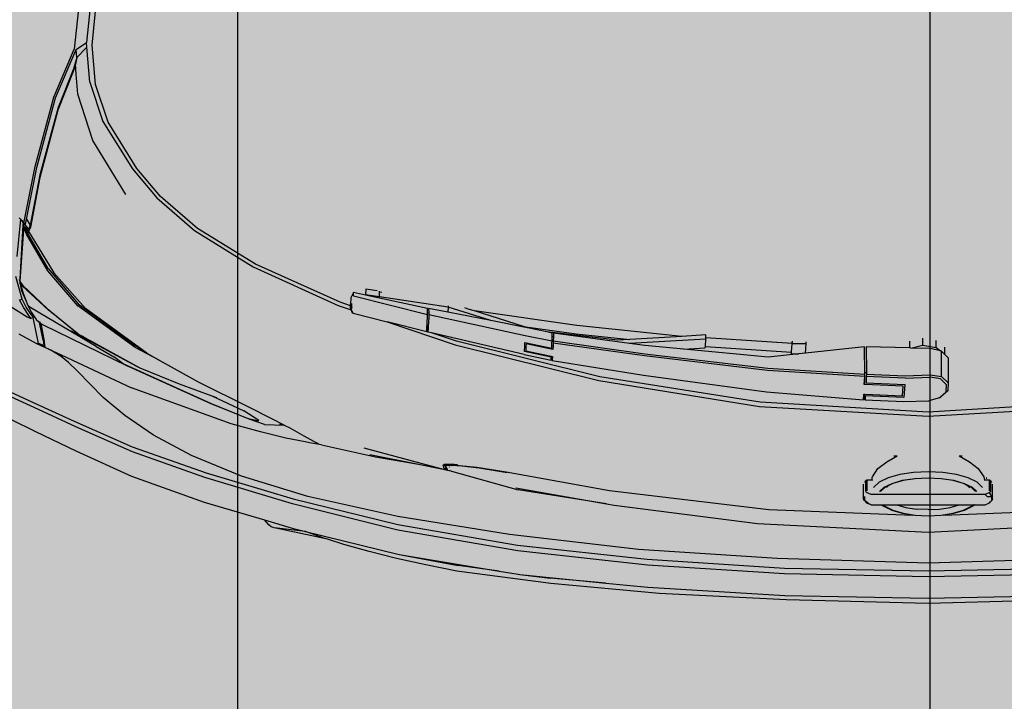
# Model space of a CAD drawing. Units: inches. Extents: x 1884 to 2398, y 474 to 1488.
# Tile 5 of 39: x 2203 to 2232, y 577 to 597. Entities that reach past the tile are written whole.
import ezdxf

# ---------------------------------------------------------------- set-up
doc = ezdxf.new("R2010")
doc.units = ezdxf.units.IN
doc.header["$MEASUREMENT"] = 0
doc.layers.get('0').update_dxf_attribs({"color": 250})
doc.layers.add('A-ANNO-DIMS', color=2, linetype='Continuous', lineweight=18)
doc.layers.add('C-VEHI', color=8, linetype='Continuous', lineweight=18)
doc.layers.add('Edges', color=250, linetype='Continuous')
doc.layers.add('L-PVMT-PATT', color=9, linetype='Continuous', lineweight=13, true_color=0xc7c8ca)
doc.styles.get("Standard").update_dxf_attribs({"font": 'arial.ttf'})
doc.dimstyles.get("Standard").update_dxf_attribs({"dimtxt": 7, "dimasz": 0.18, "dimexe": 0.18, "dimexo": 0.0625, "dimgap": 0.09, "dimtad": 0, "dimtih": 1, "dimtoh": 1, "dimzin": 0, "dimdsep": 46, "dimlunit": 3, "dimtxsty": 'Standard', "dimcen": 0.09, "dimadec": 0, "dimazin": 0, "dimtfac": 1, "dimtofl": 0, "dimtmove": 0, "dimatfit": 3, "dimfxl": 1, "dimtolj": 1, "dimtzin": 0, "dimarcsym": 0})

# ---------------------------------------------------------------- blocks, each defined once
blk = doc.blocks.new('Nissan Qashqai pl')
at = {"layer": 'Edges'}
for p, q in [((11.5166, 12.04708), (11.52386, 11.92208)), ((11.52698, 11.92208), (11.51964, 12.0475)), ((11.61327, 11.92208), (11.60675, 12.04892)), ((11.60051, 11.93346), (11.59629, 12.04057)), ((11.63292, 12.0344), (11.63628, 11.92208)), ((11.64211, 11.92208), (11.63993, 12.02899)), ((11.64437, 12.02886), (11.64655, 11.92208)), ((11.66226, 11.92208), (11.66041, 12.02874)), ((11.66349, 12.02738), (11.66628, 11.92208)), ((11.57479, 11.96843), (11.57457, 11.96768)), ((11.58239, 11.96768), (11.57457, 11.96768)), ((11.57457, 11.96768), (11.57457, 11.96395)), ((11.57617, 11.96938), (11.57479, 11.96843)), ((11.57479, 11.96843), (11.58262, 11.96843)), ((11.58846, 11.97008), (11.57758, 11.97008)), ((11.58262, 11.96843), (11.58377, 11.96782)), ((11.58668, 11.96947), (11.58377, 11.96782)), ((11.58377, 11.96782), (11.58513, 11.96453)), ((11.58679, 11.96604), (11.58668, 11.96947)), ((11.58961, 11.96947), (11.58668, 11.96947)), ((11.58846, 11.97008), (11.58961, 11.96947)), ((11.5915, 11.96782), (11.58961, 11.96947)), ((11.5915, 11.96782), (11.59043, 11.96839)), ((11.59285, 11.96453), (11.5915, 11.96782)), ((11.56082, 11.95281), (11.56588, 11.95938)), ((11.56588, 11.95938), (11.57195, 11.96347)), ((11.57195, 11.96347), (11.57457, 11.96395)), ((11.57261, 11.96533), (11.57261, 11.96561)), ((11.57306, 11.96528), (11.57306, 11.96569)), ((11.57457, 11.96395), (11.57457, 11.96378)), ((11.57994, 11.96265), (11.57613, 11.95845)), ((11.58679, 11.96604), (11.58513, 11.96453)), ((11.58513, 11.96453), (11.58513, 11.87963)), ((11.59285, 11.95694), (11.59285, 11.96453)), ((11.55816, 11.94815), (11.56082, 11.95281)), ((11.57286, 11.95178), (11.57035, 11.94308)), ((11.57613, 11.95845), (11.57286, 11.95178)), ((11.57692, 11.94885), (11.57987, 11.95487)), ((11.57876, 11.95169), (11.57712, 11.94834)), ((11.58001, 11.95424), (11.57876, 11.95169)), ((11.57876, 11.95169), (11.57995, 11.953)), ((11.57987, 11.95487), (11.58291, 11.95821)), ((11.58291, 11.95743), (11.58001, 11.95424)), ((11.59285, 11.95694), (11.59412, 11.95487)), ((11.59285, 11.95657), (11.59285, 11.95694)), ((11.59319, 11.9559), (11.59285, 11.95657)), ((11.59285, 11.95626), (11.59285, 11.95657)), ((11.59285, 11.95626), (11.59319, 11.9559)), ((11.59285, 11.95549), (11.59285, 11.95626)), ((11.59398, 11.95424), (11.59285, 11.95549)), ((11.59285, 11.94526), (11.59285, 11.95549)), ((11.59319, 11.9559), (11.59412, 11.95487)), ((11.59688, 11.94834), (11.59398, 11.95424)), ((11.59412, 11.95487), (11.59707, 11.94885)), ((11.55654, 11.94509), (11.55639, 11.94749)), ((11.55654, 11.94509), (11.55816, 11.94815)), ((11.57466, 11.94101), (11.57692, 11.94885)), ((11.57712, 11.94834), (11.5749, 11.94065)), ((11.59285, 11.8989), (11.59285, 11.94526)), ((11.59478, 11.93858), (11.59285, 11.94526)), ((11.5991, 11.94065), (11.59688, 11.94834)), ((11.59707, 11.94885), (11.59933, 11.94101)), ((11.48349, 11.93703), (11.48106, 11.93457)), ((11.48349, 11.93703), (11.50222, 11.93704)), ((11.49744, 11.93207), (11.50222, 11.93704)), ((11.50222, 11.93704), (11.50812, 11.93671)), ((11.57035, 11.94308), (11.56877, 11.93295)), ((11.57324, 11.93188), (11.57466, 11.94101)), ((11.5749, 11.94065), (11.5735, 11.93169)), ((11.59602, 11.93062), (11.59478, 11.93858)), ((11.60049, 11.93169), (11.5991, 11.94065)), ((11.59933, 11.94101), (11.60051, 11.93346)), ((11.48106, 11.93457), (11.47554, 11.93456)), ((11.47578, 11.92803), (11.4784, 11.93124)), ((11.4784, 11.93124), (11.47657, 11.92368)), ((11.4786, 11.93206), (11.4784, 11.93124)), ((11.48106, 11.93457), (11.4786, 11.93206)), ((11.49744, 11.93207), (11.4786, 11.93206)), ((11.49621, 11.92369), (11.49744, 11.93207)), ((11.49907, 11.93132), (11.49795, 11.92364)), ((11.50349, 11.93588), (11.49907, 11.93132)), ((11.50889, 11.93558), (11.50349, 11.93588)), ((11.50812, 11.93671), (11.51287, 11.9312)), ((11.50889, 11.93558), (11.51321, 11.93053)), ((11.51321, 11.93053), (11.51287, 11.9312)), ((11.51321, 11.93053), (11.51543, 11.92267)), ((11.56877, 11.93295), (11.56823, 11.92208)), ((11.57275, 11.92208), (11.57324, 11.93188)), ((11.5735, 11.93169), (11.57302, 11.92208)), ((11.59645, 11.92208), (11.59602, 11.93062)), ((11.60097, 11.92208), (11.60049, 11.93169)), ((11.60051, 11.93346), (11.60076, 11.93188)), ((11.60076, 11.93188), (11.60124, 11.92208)), ((11.47578, 11.92803), (11.47062, 11.92803)), ((11.47398, 11.91798), (11.47578, 11.92803)), ((11.47657, 11.92368), (11.47622, 11.90912)), ((11.49689, 11.90495), (11.49621, 11.92369)), ((11.49859, 11.9049), (11.49795, 11.92364)), ((11.51606, 11.90392), (11.51543, 11.92267)), ((11.46896, 11.91798), (11.47398, 11.91798)), ((11.47622, 11.90912), (11.47398, 11.91798)), ((11.52386, 11.92208), (11.5166, 11.79708)), ((11.51964, 11.79666), (11.52698, 11.92208)), ((11.56823, 11.92208), (11.56877, 11.91121)), ((11.57324, 11.91228), (11.57275, 11.92208)), ((11.57302, 11.92208), (11.5735, 11.91247)), ((11.59645, 11.92208), (11.59602, 11.91354)), ((11.60049, 11.91247), (11.60097, 11.92208)), ((11.60124, 11.92208), (11.60076, 11.91228)), ((11.60675, 11.79524), (11.61327, 11.92208)), ((11.63628, 11.92208), (11.63292, 11.80976)), ((11.63993, 11.81518), (11.64211, 11.92208)), ((11.64655, 11.92208), (11.64437, 11.8153)), ((11.66041, 11.81542), (11.66226, 11.92208)), ((11.66628, 11.92208), (11.66349, 11.81678)), ((11.47102, 11.90825), (11.4762, 11.90826)), ((11.4762, 11.90826), (11.47542, 11.87608)), ((11.47622, 11.90912), (11.4762, 11.90826)), ((11.56877, 11.91121), (11.57035, 11.90108)), ((11.57466, 11.90315), (11.57324, 11.91228)), ((11.5735, 11.91247), (11.5749, 11.90351)), ((11.59478, 11.90558), (11.59602, 11.91354)), ((11.59629, 11.80359), (11.60051, 11.91071)), ((11.5991, 11.90351), (11.60049, 11.91247)), ((11.60051, 11.91071), (11.59933, 11.90315)), ((11.60076, 11.91228), (11.60051, 11.91071)), ((11.49565, 11.87616), (11.49689, 11.90495)), ((11.49859, 11.9049), (11.49735, 11.87612)), ((11.50223, 11.8759), (11.50346, 11.90468)), ((11.50462, 11.90341), (11.50341, 11.87505)), ((11.50346, 11.90468), (11.51299, 11.90415)), ((11.51177, 11.90301), (11.50462, 11.90341)), ((11.51058, 11.87508), (11.51177, 11.90301)), ((11.51299, 11.90415), (11.51176, 11.87537)), ((11.51483, 11.87514), (11.51606, 11.90392)), ((11.57035, 11.90108), (11.57286, 11.89238)), ((11.57692, 11.89531), (11.57466, 11.90315)), ((11.5749, 11.90351), (11.57712, 11.89582)), ((11.59285, 11.8989), (11.59478, 11.90558)), ((11.59688, 11.89582), (11.5991, 11.90351)), ((11.59933, 11.90315), (11.59707, 11.89531)), ((11.55639, 11.89667), (11.55654, 11.89907)), ((11.55816, 11.89601), (11.55654, 11.89907)), ((11.56082, 11.89135), (11.55816, 11.89601)), ((11.57987, 11.88929), (11.57692, 11.89531)), ((11.57712, 11.89582), (11.57876, 11.89248)), ((11.59285, 11.88868), (11.59285, 11.8989)), ((11.59398, 11.88992), (11.59688, 11.89582)), ((11.59707, 11.89531), (11.59412, 11.88929)), ((11.56588, 11.88478), (11.56082, 11.89135)), ((11.57286, 11.89238), (11.57613, 11.88571)), ((11.57995, 11.89116), (11.57876, 11.89248)), ((11.57876, 11.89248), (11.58001, 11.88992)), ((11.58291, 11.88595), (11.57987, 11.88929)), ((11.58001, 11.88992), (11.58291, 11.88673)), ((11.59285, 11.88868), (11.59398, 11.88992)), ((11.59285, 11.88722), (11.59412, 11.88929)), ((11.59285, 11.8879), (11.59285, 11.88868)), ((11.59285, 11.88759), (11.59319, 11.88827)), ((11.59319, 11.88827), (11.59285, 11.8879)), ((11.59285, 11.88759), (11.59285, 11.8879)), ((11.59285, 11.88722), (11.59285, 11.88759)), ((11.59285, 11.87963), (11.59285, 11.88722)), ((11.59412, 11.88929), (11.59319, 11.88827)), ((11.57195, 11.88069), (11.56588, 11.88478)), ((11.57261, 11.88057), (11.57195, 11.88069)), ((11.57261, 11.88057), (11.57261, 11.88076)), ((11.57306, 11.88049), (11.57261, 11.88057)), ((11.57306, 11.88049), (11.57306, 11.88081)), ((11.57457, 11.88021), (11.57306, 11.88049)), ((11.57457, 11.88096), (11.57457, 11.88021)), ((11.57457, 11.88021), (11.57457, 11.87648)), ((11.57613, 11.88571), (11.57994, 11.88151)), ((11.58513, 11.87963), (11.58377, 11.87635)), ((11.59285, 11.87963), (11.59221, 11.87812)), ((11.49563, 11.87496), (11.47539, 11.87488)), ((11.47539, 11.87488), (11.4801, 11.83099)), ((11.47542, 11.87608), (11.49451, 11.87616)), ((11.49133, 11.80278), (11.49563, 11.87496)), ((11.49732, 11.87492), (11.49295, 11.80271)), ((11.49449, 11.87502), (11.49451, 11.87616)), ((11.50341, 11.87505), (11.49449, 11.87502)), ((11.49451, 11.87616), (11.49565, 11.87616)), ((11.49732, 11.87492), (11.49563, 11.87496)), ((11.49565, 11.87616), (11.49735, 11.87612)), ((11.50339, 11.87463), (11.49732, 11.87492)), ((11.49735, 11.87612), (11.50223, 11.8759)), ((11.50341, 11.87505), (11.50339, 11.87463)), ((11.50884, 11.80182), (11.5148, 11.87394)), ((11.51054, 11.87423), (11.51058, 11.87508)), ((11.5148, 11.87394), (11.51054, 11.87423)), ((11.51472, 11.8751), (11.51058, 11.87508)), ((11.51176, 11.87537), (11.51472, 11.87515)), ((11.51472, 11.87515), (11.51472, 11.8751)), ((11.51472, 11.87515), (11.51483, 11.87514)), ((11.51483, 11.87514), (11.51472, 11.8751)), ((11.57457, 11.87648), (11.58239, 11.87648)), ((11.57457, 11.87648), (11.57479, 11.87573)), ((11.58262, 11.87573), (11.57479, 11.87573)), ((11.57479, 11.87573), (11.57617, 11.87478)), ((11.58846, 11.87408), (11.57758, 11.87408)), ((11.58377, 11.87635), (11.58262, 11.87573)), ((11.58668, 11.87469), (11.58961, 11.87469)), ((11.58961, 11.87469), (11.58846, 11.87408)), ((11.58961, 11.87469), (11.5915, 11.87635)), ((11.59043, 11.87577), (11.58961, 11.87469)), ((11.59221, 11.87812), (11.59043, 11.87577)), ((11.59043, 11.87577), (11.5915, 11.87635)), ((11.5915, 11.87635), (11.59221, 11.87812)), ((11.47305, 11.83139), (11.47165, 11.83144)), ((11.47305, 11.83139), (11.473, 11.82087)), ((11.4801, 11.83099), (11.47305, 11.83139)), ((11.4801, 11.83099), (11.48065, 11.82584)), ((11.47281, 11.82086), (11.46872, 11.75675)), ((11.47111, 11.82093), (11.47189, 11.82089)), ((11.47281, 11.82086), (11.47189, 11.82089)), ((11.473, 11.82087), (11.47281, 11.82086)), ((11.47916, 11.8205), (11.473, 11.82087)), ((11.47508, 11.75641), (11.47919, 11.82046)), ((11.47919, 11.82046), (11.47916, 11.8205)), ((11.48062, 11.82044), (11.47919, 11.82046)), ((11.48062, 11.82044), (11.48065, 11.82584)), ((11.48065, 11.82584), (11.4831, 11.803)), ((11.63327, 11.71316), (11.63993, 11.81518)), ((11.64437, 11.8153), (11.63768, 11.7134)), ((11.65425, 11.71357), (11.66041, 11.81542)), ((11.66349, 11.81678), (11.65888, 11.72193)), ((11.63292, 11.80976), (11.62604, 11.70665)), ((11.4831, 11.803), (11.47707, 11.74042)), ((11.4805, 11.71128), (11.49133, 11.80278)), ((11.49295, 11.80271), (11.48212, 11.71121)), ((11.49642, 11.71041), (11.50884, 11.80182)), ((11.58235, 11.68521), (11.59629, 11.80359)), ((11.5166, 11.79708), (11.49761, 11.67796)), ((11.50045, 11.6772), (11.51964, 11.79666)), ((11.5932, 11.68852), (11.60675, 11.79524)), ((11.46872, 11.75675), (11.46649, 11.75682)), ((11.46649, 11.75682), (11.46757, 11.73891)), ((11.46975, 11.75671), (11.46872, 11.75675)), ((11.46975, 11.75671), (11.47273, 11.69994)), ((11.47508, 11.75641), (11.46975, 11.75671)), ((11.47611, 11.75636), (11.47508, 11.75641)), ((11.47707, 11.74042), (11.47611, 11.75636)), ((11.47707, 11.74042), (11.47428, 11.71144)), ((11.46757, 11.73891), (11.45941, 11.6607)), ((11.46757, 11.73891), (11.46992, 11.70014)), ((11.65888, 11.72193), (11.65143, 11.64152)), ((11.47094, 11.64327), (11.4805, 11.71128)), ((11.48212, 11.71121), (11.47257, 11.6432)), ((11.47428, 11.71144), (11.47273, 11.69994)), ((11.48539, 11.64249), (11.49642, 11.71041)), ((11.6229, 11.61679), (11.63327, 11.71316)), ((11.63768, 11.7134), (11.62719, 11.61693)), ((11.65114, 11.68233), (11.65425, 11.71357)), ((11.62604, 11.70665), (11.61495, 11.61084)), ((11.47273, 11.69994), (11.46512, 11.64343)), ((11.46576, 11.66035), (11.46992, 11.70014)), ((11.46992, 11.70014), (11.47047, 11.69095)), ((11.47047, 11.69095), (11.46419, 11.63849)), ((11.59218, 11.68277), (11.5932, 11.68852)), ((11.56846, 11.60829), (11.58235, 11.68521)), ((11.58021, 11.61555), (11.59218, 11.68277)), ((11.59218, 11.68277), (11.58179, 11.61717)), ((11.64478, 11.61839), (11.65114, 11.68233)), ((11.65114, 11.68233), (11.64749, 11.64092)), ((11.49761, 11.67796), (11.47115, 11.57128)), ((11.47375, 11.5702), (11.50045, 11.6772)), ((11.45941, 11.6607), (11.44866, 11.58459)), ((11.46024, 11.62121), (11.46576, 11.66035)), ((11.46419, 11.63849), (11.46114, 11.62406)), ((11.46505, 11.64255), (11.46419, 11.63849)), ((11.46792, 11.64248), (11.46505, 11.64255)), ((11.46512, 11.64343), (11.46801, 11.64335)), ((11.46687, 11.62247), (11.47088, 11.64239)), ((11.46801, 11.64335), (11.46792, 11.64248)), ((11.47088, 11.64239), (11.46792, 11.64248)), ((11.46801, 11.64335), (11.47094, 11.64327)), ((11.47252, 11.64233), (11.47088, 11.64239)), ((11.47094, 11.64327), (11.47257, 11.6432)), ((11.47212, 11.62223), (11.47625, 11.64214)), ((11.47439, 11.64223), (11.47252, 11.64233)), ((11.47257, 11.6432), (11.47449, 11.6431)), ((11.47727, 11.64296), (11.47315, 11.62305)), ((11.47439, 11.64223), (11.47449, 11.6431)), ((11.47625, 11.64214), (11.47439, 11.64223)), ((11.47449, 11.6431), (11.47727, 11.64296)), ((11.47827, 11.62277), (11.48226, 11.64167)), ((11.48298, 11.64165), (11.47879, 11.62186)), ((11.48098, 11.62171), (11.48532, 11.64161)), ((11.48226, 11.64167), (11.48244, 11.64254)), ((11.48226, 11.64167), (11.48298, 11.64165)), ((11.48244, 11.64254), (11.48247, 11.64267)), ((11.48535, 11.64246), (11.48244, 11.64254)), ((11.48247, 11.64267), (11.48535, 11.64246)), ((11.483, 11.64176), (11.48298, 11.64165)), ((11.48532, 11.64161), (11.483, 11.64176)), ((11.48539, 11.64249), (11.48535, 11.64246)), ((11.65143, 11.64152), (11.64217, 11.57162)), ((11.64478, 11.61839), (11.64749, 11.64092)), ((11.45125, 11.55073), (11.46687, 11.62247)), ((11.46083, 11.62261), (11.45585, 11.5969)), ((11.46114, 11.62406), (11.46024, 11.62121)), ((11.46114, 11.62406), (11.46083, 11.62261)), ((11.47495, 11.62207), (11.47212, 11.62223)), ((11.47315, 11.62305), (11.47515, 11.62294)), ((11.47495, 11.62207), (11.47515, 11.62294)), ((11.47515, 11.62294), (11.47827, 11.62277)), ((11.46024, 11.62121), (11.44866, 11.58459)), ((11.48098, 11.62171), (11.4649, 11.55261)), ((11.47879, 11.62186), (11.47495, 11.62207)), ((11.56776, 11.56755), (11.58179, 11.61717)), ((11.60765, 11.5276), (11.6229, 11.61679)), ((11.62719, 11.61693), (11.61178, 11.52762)), ((11.64227, 11.603), (11.64462, 11.61709)), ((11.64462, 11.61709), (11.64478, 11.61839)), ((11.56499, 11.58644), (11.56846, 11.60829)), ((11.56905, 11.60888), (11.56563, 11.58822)), ((11.61495, 11.61084), (11.6016, 11.52761)), ((11.63012, 11.53004), (11.64227, 11.603)), ((11.64227, 11.603), (11.63807, 11.5726)), ((11.45585, 11.5969), (11.44582, 11.56516)), ((11.45585, 11.5969), (11.44965, 11.56495)), ((11.56356, 11.57357), (11.56499, 11.58644)), ((11.56563, 11.58822), (11.56415, 11.57536)), ((11.44723, 11.58007), (11.44639, 11.57739)), ((11.44866, 11.58459), (11.44723, 11.58007)), ((11.47115, 11.57128), (11.4649, 11.55261)), ((11.56268, 11.56956), (11.5628, 11.57206)), ((11.56335, 11.56843), (11.56356, 11.57357)), ((11.56415, 11.57536), (11.56375, 11.56794)), ((11.63012, 11.53004), (11.63807, 11.5726)), ((11.64217, 11.57162), (11.63751, 11.54857)), ((11.44575, 11.56516), (11.43801, 11.51398)), ((11.4448, 11.5652), (11.44575, 11.56516)), ((11.44575, 11.56516), (11.44582, 11.56516)), ((11.44582, 11.56516), (11.44965, 11.56495)), ((11.44965, 11.56495), (11.44685, 11.5505)), ((11.45676, 11.51971), (11.47375, 11.5702)), ((11.56255, 11.56701), (11.56268, 11.56956)), ((11.56271, 11.56245), (11.56255, 11.56701)), ((11.56268, 11.56956), (11.56259, 11.5697)), ((11.56335, 11.56843), (11.56268, 11.56956)), ((11.56325, 11.56586), (11.56335, 11.56843)), ((11.56334, 11.56271), (11.56325, 11.56586)), ((11.56609, 11.56386), (11.56334, 11.56271)), ((11.56368, 11.56788), (11.56335, 11.56843)), ((11.56375, 11.56794), (11.56392, 11.56325)), ((11.56429, 11.56338), (11.56596, 11.56408)), ((11.56487, 11.5659), (11.56469, 11.5662)), ((11.56609, 11.56386), (11.56583, 11.56223)), ((11.56596, 11.56408), (11.56616, 11.56417)), ((11.56609, 11.56386), (11.56596, 11.56408)), ((11.56613, 11.56388), (11.56609, 11.56386)), ((11.56618, 11.56418), (11.56613, 11.56388)), ((11.56613, 11.56388), (11.56616, 11.56417)), ((11.56613, 11.56388), (11.56645, 11.5641)), ((11.56665, 11.56424), (11.56616, 11.56236)), ((11.56616, 11.56417), (11.56618, 11.56418)), ((11.56616, 11.56236), (11.56645, 11.5641)), ((11.56618, 11.56418), (11.56648, 11.56431)), ((11.56645, 11.5641), (11.56648, 11.56431)), ((11.56645, 11.5641), (11.56665, 11.56424)), ((11.56648, 11.56431), (11.56669, 11.5644)), ((11.56661, 11.56253), (11.56704, 11.56455)), ((11.56665, 11.56424), (11.56688, 11.56448)), ((11.56669, 11.5644), (11.56665, 11.56424)), ((11.56669, 11.5644), (11.56688, 11.56448)), ((11.56671, 11.56257), (11.56712, 11.56458)), ((11.56717, 11.5646), (11.56679, 11.56261)), ((11.56688, 11.56448), (11.56704, 11.56455)), ((11.56704, 11.56455), (11.56739, 11.56625)), ((11.56704, 11.56455), (11.56712, 11.56458)), ((11.56712, 11.56458), (11.56763, 11.56708)), ((11.56712, 11.56458), (11.56717, 11.5646)), ((11.56717, 11.5646), (11.56763, 11.56708)), ((11.56745, 11.56646), (11.56739, 11.56625)), ((11.56763, 11.56708), (11.56776, 11.56755)), ((11.55053, 11.5023), (11.56648, 11.56144)), ((11.56334, 11.56271), (11.56271, 11.56245)), ((11.56338, 11.56129), (11.56271, 11.56245)), ((11.56273, 11.5431), (11.56648, 11.56144)), ((11.56338, 11.56129), (11.56334, 11.56271)), ((11.56583, 11.56223), (11.56338, 11.56129)), ((11.56392, 11.56325), (11.56429, 11.56338)), ((11.56616, 11.56236), (11.56583, 11.56223)), ((11.56661, 11.56253), (11.56616, 11.56236)), ((11.56679, 11.56261), (11.56648, 11.56144)), ((11.56671, 11.56257), (11.56661, 11.56253)), ((11.56679, 11.56261), (11.56671, 11.56257)), ((11.43747, 11.49463), (11.45125, 11.54985)), ((11.44684, 11.54963), (11.43914, 11.51392)), ((11.44983, 11.54978), (11.44684, 11.54963)), ((11.44685, 11.5505), (11.44997, 11.55066)), ((11.44983, 11.54978), (11.44997, 11.55066)), ((11.45125, 11.54985), (11.44983, 11.54978)), ((11.44997, 11.55066), (11.45125, 11.55073)), ((11.45125, 11.55073), (11.4529, 11.55066)), ((11.4529, 11.54978), (11.45125, 11.54985)), ((11.4529, 11.55066), (11.45711, 11.55045)), ((11.45711, 11.54958), (11.4529, 11.54978)), ((11.46429, 11.54915), (11.45676, 11.51971)), ((11.45711, 11.55045), (11.45994, 11.5503)), ((11.46197, 11.5493), (11.45711, 11.54958)), ((11.45983, 11.54978), (11.45994, 11.5503)), ((11.46402, 11.54999), (11.45983, 11.54978)), ((11.45994, 11.5503), (11.46197, 11.55018)), ((11.46197, 11.55018), (11.46404, 11.55004)), ((11.46375, 11.54918), (11.46197, 11.5493)), ((11.46402, 11.54999), (11.46375, 11.54918)), ((11.46429, 11.54915), (11.46375, 11.54918)), ((11.46404, 11.55004), (11.46402, 11.54999)), ((11.46423, 11.55), (11.46402, 11.54999)), ((11.46404, 11.55004), (11.46423, 11.55)), ((11.46423, 11.55), (11.46424, 11.55003)), ((11.4643, 11.55002), (11.46423, 11.55)), ((11.4649, 11.55261), (11.4643, 11.55002)), ((11.55533, 11.50682), (11.56273, 11.5431)), ((11.55707, 11.51104), (11.56273, 11.5431)), ((11.63751, 11.54857), (11.63276, 11.52672)), ((11.6016, 11.52761), (11.58664, 11.46068)), ((11.58843, 11.44985), (11.60765, 11.5276)), ((11.61178, 11.52762), (11.59225, 11.44945)), ((11.61272, 11.45895), (11.62966, 11.52759)), ((11.62966, 11.52759), (11.63012, 11.53004)), ((11.45032, 11.49453), (11.45676, 11.51971)), ((11.63276, 11.52672), (11.62771, 11.50627)), ((11.43371, 11.51238), (11.43251, 11.50378)), ((11.43475, 11.51409), (11.43403, 11.51411)), ((11.43501, 11.51584), (11.43475, 11.51409)), ((11.43801, 11.51398), (11.43475, 11.51409)), ((11.4382, 11.51397), (11.43676, 11.50364)), ((11.43914, 11.51392), (11.43692, 11.50363)), ((11.4382, 11.51397), (11.43801, 11.51398)), ((11.43914, 11.51392), (11.4382, 11.51397)), ((11.54814, 11.47101), (11.55707, 11.51104)), ((11.62771, 11.50627), (11.62241, 11.48743)), ((11.43251, 11.50378), (11.43676, 11.50364)), ((11.43251, 11.50378), (11.4369, 11.50353)), ((11.4369, 11.50353), (11.435, 11.49469)), ((11.43676, 11.50364), (11.43692, 11.50363)), ((11.43692, 11.50363), (11.4369, 11.50353)), ((11.435, 11.49469), (11.43896, 11.49272)), ((11.43747, 11.49463), (11.435, 11.49469)), ((11.43896, 11.49272), (11.44373, 11.49245)), ((11.44474, 11.49242), (11.44218, 11.48476)), ((11.44507, 11.49341), (11.44316, 11.49351)), ((11.44373, 11.49245), (11.44491, 11.49291)), ((11.44474, 11.49242), (11.44373, 11.49245)), ((11.44453, 11.48334), (11.44778, 11.49299)), ((11.44491, 11.49291), (11.44474, 11.49242)), ((11.4462, 11.49239), (11.44474, 11.49242)), ((11.44507, 11.49341), (11.44491, 11.49291)), ((11.44491, 11.49291), (11.44606, 11.49335)), ((11.44606, 11.49335), (11.44507, 11.49341)), ((11.44786, 11.49325), (11.44606, 11.49335)), ((11.44786, 11.49325), (11.4462, 11.49239)), ((11.44778, 11.49299), (11.4462, 11.49239)), ((11.45018, 11.49392), (11.44778, 11.49299)), ((11.44794, 11.49325), (11.44786, 11.49325)), ((11.45032, 11.49453), (11.44794, 11.49325)), ((11.45018, 11.49392), (11.45032, 11.49453)), ((11.44218, 11.48476), (11.41383, 11.42186)), ((11.41588, 11.41997), (11.44453, 11.48334)), ((11.62241, 11.48743), (11.61848, 11.47528)), ((11.54554, 11.46484), (11.54721, 11.46841)), ((11.54814, 11.47101), (11.54666, 11.46197)), ((11.61848, 11.47528), (11.61008, 11.43562)), ((11.61742, 11.47198), (11.61272, 11.45895)), ((11.61848, 11.47528), (11.61742, 11.47198)), ((11.54162, 11.45783), (11.54554, 11.46484)), ((11.54666, 11.46197), (11.54611, 11.45874)), ((11.53572, 11.44731), (11.54162, 11.45783)), ((11.54611, 11.45874), (11.54336, 11.44449)), ((11.58664, 11.46068), (11.57152, 11.41151)), ((11.61272, 11.45895), (11.61008, 11.43562)), ((11.61028, 11.44915), (11.61272, 11.45895)), ((11.53354, 11.44315), (11.53572, 11.44731)), ((11.56912, 11.38501), (11.58843, 11.44985)), ((11.59225, 11.44945), (11.57263, 11.38419)), ((11.60419, 11.42861), (11.61028, 11.44915)), ((11.52833, 11.43321), (11.53335, 11.4428)), ((11.53261, 11.43965), (11.5333, 11.44225)), ((11.53313, 11.42848), (11.53354, 11.44315)), ((11.5333, 11.44225), (11.53335, 11.4428)), ((11.53335, 11.4428), (11.53354, 11.44315)), ((11.54336, 11.44449), (11.53855, 11.42543)), ((11.5202, 11.41712), (11.52833, 11.43321)), ((11.60938, 11.43347), (11.60772, 11.43162)), ((11.61008, 11.43562), (11.60938, 11.43347)), ((11.53009, 11.42439), (11.52299, 11.41307)), ((11.53313, 11.42848), (11.52922, 11.417)), ((11.53022, 11.42324), (11.53009, 11.42439)), ((11.53855, 11.42543), (11.53253, 11.4038)), ((11.59084, 11.38361), (11.60419, 11.42861)), ((11.60772, 11.43162), (11.60419, 11.42861)), ((11.41383, 11.42186), (11.38718, 11.37878)), ((11.38877, 11.37638), (11.41588, 11.41997)), ((11.50131, 11.37908), (11.5202, 11.41712)), ((11.52855, 11.41625), (11.53022, 11.42324)), ((11.5118, 11.38938), (11.52299, 11.41307)), ((11.52922, 11.417), (11.51787, 11.38901)), ((11.51787, 11.38901), (11.52855, 11.41625)), ((11.57152, 11.41151), (11.55624, 11.37411)), ((11.53253, 11.4038), (11.50574, 11.32965)), ((11.51787, 11.38901), (11.48801, 11.32337)), ((11.49005, 11.3275), (11.51787, 11.38901)), ((11.50277, 11.36495), (11.5118, 11.38938)), ((11.5118, 11.38938), (11.51304, 11.39274)), ((11.54963, 11.33002), (11.56912, 11.38501)), ((11.57263, 11.38419), (11.5535, 11.33028)), ((11.57164, 11.32969), (11.59084, 11.38361)), ((11.38718, 11.37878), (11.3635, 11.35125)), ((11.36451, 11.34835), (11.38877, 11.37638)), ((11.48518, 11.35017), (11.50131, 11.37908)), ((11.55624, 11.37411), (11.54097, 11.34593)), ((11.49086, 11.33567), (11.50277, 11.36495)), ((11.3635, 11.35125), (11.34251, 11.3336)), ((11.34283, 11.33026), (11.36451, 11.34835)), ((11.48518, 11.35017), (11.4758, 11.33232)), ((11.48012, 11.34111), (11.48518, 11.35017)), ((11.54097, 11.34593), (11.52646, 11.32473)), ((11.48005, 11.341), (11.44669, 11.29536)), ((11.47876, 11.33901), (11.47454, 11.33252)), ((11.47876, 11.33901), (11.48005, 11.341)), ((11.48005, 11.341), (11.48012, 11.34111)), ((11.30757, 11.30833), (11.34283, 11.33026)), ((11.34251, 11.3336), (11.3082, 11.31215)), ((11.44331, 11.28988), (11.47454, 11.33252)), ((11.4758, 11.33232), (11.44474, 11.28965)), ((11.46332, 11.28473), (11.48966, 11.33337)), ((11.47038, 11.29841), (11.49086, 11.33567)), ((11.47038, 11.29841), (11.48966, 11.33337)), ((11.48133, 11.27727), (11.50574, 11.32965)), ((11.48966, 11.33337), (11.49086, 11.33567)), ((11.53062, 11.28691), (11.54963, 11.33002)), ((11.5535, 11.33028), (11.53487, 11.28826)), ((11.55274, 11.28821), (11.57164, 11.32969)), ((11.36192, 11.32544), (11.32179, 11.30083)), ((11.45883, 11.26345), (11.48954, 11.32636)), ((11.48801, 11.32337), (11.48281, 11.31653)), ((11.48983, 11.32694), (11.48954, 11.32636)), ((11.48983, 11.32694), (11.49005, 11.3275)), ((11.52646, 11.32473), (11.51313, 11.30854)), ((11.47499, 11.30324), (11.48281, 11.31653)), ((11.27848, 11.29865), (11.30757, 11.30833)), ((11.3082, 11.31215), (11.28005, 11.30276)), ((11.51313, 11.30854), (11.49329, 11.28912)), ((11.2509, 11.3003), (11.21523, 11.3038)), ((11.28005, 11.30276), (11.2509, 11.3003)), ((11.32179, 11.30083), (11.28736, 11.28974)), ((11.47499, 11.30324), (11.4462, 11.25482)), ((11.21271, 11.29983), (11.24875, 11.29618)), ((11.25238, 11.29648), (11.24875, 11.29618)), ((11.2541, 11.28846), (11.24875, 11.29618)), ((11.27848, 11.29865), (11.25238, 11.29648)), ((11.25238, 11.29648), (11.25993, 11.28891)), ((11.42028, 11.27173), (11.44669, 11.29536)), ((11.46587, 11.29022), (11.46737, 11.29293)), ((11.46746, 11.29312), (11.46737, 11.29293)), ((11.46746, 11.29312), (11.47026, 11.29821)), ((11.47026, 11.29821), (11.47038, 11.29841)), ((11.21656, 11.2908), (11.25377, 11.28706)), ((11.25857, 11.28503), (11.25377, 11.28706)), ((11.25993, 11.28891), (11.2541, 11.28846)), ((11.29, 11.2731), (11.2541, 11.28846)), ((11.25993, 11.28891), (11.25999, 11.28889)), ((11.25999, 11.28889), (11.26503, 11.28789)), ((11.25999, 11.28889), (11.26771, 11.28668)), ((11.27242, 11.28847), (11.26503, 11.28789)), ((11.26503, 11.28789), (11.27055, 11.28622)), ((11.26771, 11.28668), (11.26785, 11.28663)), ((11.26785, 11.28663), (11.29721, 11.27493)), ((11.27055, 11.28622), (11.29928, 11.27468)), ((11.28736, 11.28974), (11.27242, 11.28847)), ((11.41708, 11.26758), (11.44331, 11.28988)), ((11.44474, 11.28965), (11.41866, 11.26734)), ((11.44691, 11.26684), (11.46587, 11.29022)), ((11.46538, 11.28932), (11.44788, 11.2676)), ((11.46538, 11.28932), (11.46587, 11.29022)), ((11.49329, 11.28912), (11.48692, 11.28262)), ((11.51652, 11.25601), (11.53062, 11.28691)), ((11.53487, 11.28826), (11.52058, 11.25724)), ((11.53843, 11.2583), (11.55274, 11.28821)), ((11.28951, 11.27177), (11.25857, 11.28503)), ((11.48133, 11.27727), (11.48217, 11.27864)), ((11.48692, 11.28262), (11.48256, 11.27724)), ((11.3411, 11.25789), (11.28951, 11.27177)), ((11.34188, 11.25916), (11.29, 11.2731)), ((11.29721, 11.27493), (11.34742, 11.26142)), ((11.29928, 11.27468), (11.34932, 11.2614)), ((11.39234, 11.25471), (11.42028, 11.27173)), ((11.47707, 11.26812), (11.48133, 11.27727)), ((11.48256, 11.27724), (11.47783, 11.26953)), ((11.41708, 11.26758), (11.38507, 11.24911)), ((11.41866, 11.26734), (11.3914, 11.25156)), ((11.42958, 11.2488), (11.44691, 11.26684)), ((11.44788, 11.2676), (11.43028, 11.24852)), ((11.47041, 11.26385), (11.45732, 11.2612)), ((11.45781, 11.262), (11.45883, 11.26345)), ((11.46049, 11.26254), (11.47129, 11.26473)), ((11.47041, 11.26385), (11.47423, 11.26446)), ((11.47129, 11.26473), (11.47442, 11.26498)), ((11.47463, 11.26457), (11.47278, 11.2604)), ((11.47423, 11.26446), (11.47278, 11.2604)), ((11.47585, 11.26509), (11.47322, 11.2592)), ((11.47423, 11.26446), (11.47445, 11.26449)), ((11.47442, 11.26498), (11.47433, 11.26475)), ((11.47442, 11.26498), (11.47446, 11.26498)), ((11.47445, 11.26477), (11.47446, 11.26498)), ((11.47463, 11.26457), (11.47445, 11.26449)), ((11.47446, 11.26498), (11.47482, 11.26501)), ((11.47585, 11.26509), (11.47463, 11.26457)), ((11.47482, 11.26501), (11.47475, 11.26484)), ((11.47482, 11.26501), (11.47585, 11.26509)), ((11.47588, 11.26517), (11.47585, 11.26509)), ((11.47783, 11.26953), (11.47588, 11.26517)), ((11.47707, 11.26812), (11.47588, 11.26517)), ((11.37955, 11.25028), (11.3411, 11.25789)), ((11.38043, 11.25154), (11.34188, 11.25916)), ((11.34742, 11.26142), (11.38475, 11.2543)), ((11.34932, 11.2614), (11.38634, 11.25437)), ((11.44984, 11.25529), (11.45491, 11.25868)), ((11.44984, 11.25529), (11.45351, 11.25651)), ((11.45121, 11.25489), (11.45351, 11.25651)), ((11.45316, 11.25595), (11.45351, 11.25651)), ((11.47278, 11.2604), (11.45351, 11.25651)), ((11.45351, 11.25651), (11.45421, 11.25473)), ((11.45491, 11.25868), (11.45678, 11.26054)), ((11.4564, 11.26086), (11.45669, 11.26088)), ((11.45652, 11.26104), (11.45688, 11.26111)), ((11.45678, 11.26054), (11.45714, 11.2609)), ((11.45714, 11.2609), (11.45732, 11.2612)), ((11.45729, 11.26188), (11.45734, 11.2619)), ((11.45732, 11.2612), (11.45781, 11.262)), ((11.45736, 11.26195), (11.45734, 11.2619)), ((11.45736, 11.26195), (11.45755, 11.26195)), ((11.45781, 11.262), (11.46047, 11.26254)), ((11.46047, 11.26254), (11.46049, 11.26254)), ((11.47322, 11.2592), (11.46579, 11.24614)), ((11.47197, 11.25711), (11.47177, 11.25676)), ((11.47269, 11.26007), (11.47281, 11.2603)), ((11.47278, 11.2604), (11.47281, 11.2603)), ((11.47281, 11.2603), (11.47317, 11.26096)), ((11.47281, 11.2603), (11.47322, 11.2592)), ((11.50736, 11.23616), (11.51652, 11.25601)), ((11.52058, 11.25724), (11.51126, 11.23721)), ((11.52949, 11.24004), (11.53843, 11.2583)), ((11.38338, 11.24949), (11.37955, 11.25028)), ((11.38041, 11.24692), (11.38275, 11.24887)), ((11.38043, 11.25154), (11.38475, 11.2543)), ((11.38408, 11.25081), (11.38043, 11.25154)), ((11.38129, 11.24847), (11.38167, 11.2488)), ((11.38275, 11.24887), (11.38338, 11.24949)), ((11.38295, 11.24897), (11.38801, 11.25321)), ((11.38446, 11.24984), (11.38295, 11.24897)), ((11.38295, 11.24897), (11.38491, 11.2491)), ((11.38295, 11.24897), (11.38461, 11.24885)), ((11.38408, 11.25081), (11.38338, 11.24949)), ((11.38461, 11.24885), (11.38464, 11.24887)), ((11.38461, 11.24885), (11.38934, 11.2486)), ((11.38464, 11.24887), (11.38501, 11.24911)), ((11.38491, 11.2491), (11.38464, 11.24887)), ((11.38475, 11.2543), (11.38801, 11.25321)), ((11.38823, 11.2519), (11.38491, 11.2491)), ((11.38501, 11.24911), (11.38507, 11.24911)), ((11.38507, 11.24911), (11.3867, 11.24922)), ((11.38811, 11.25194), (11.3861, 11.25078)), ((11.38634, 11.25437), (11.38953, 11.25299)), ((11.3914, 11.25156), (11.3867, 11.24922)), ((11.3867, 11.24922), (11.3915, 11.24906)), ((11.38862, 11.25223), (11.38822, 11.252)), ((11.38862, 11.25223), (11.38823, 11.2519)), ((11.39063, 11.25338), (11.38862, 11.25223)), ((11.38953, 11.25299), (11.38862, 11.25223)), ((11.38953, 11.25299), (11.39234, 11.25471)), ((11.3915, 11.24906), (11.42659, 11.2465)), ((11.41698, 11.19425), (11.45295, 11.25195)), ((11.42684, 11.24649), (11.42958, 11.2488)), ((11.42996, 11.24721), (11.43609, 11.24937)), ((11.4397, 11.25049), (11.43368, 11.248)), ((11.43609, 11.24937), (11.44061, 11.25095)), ((11.44061, 11.25095), (11.4397, 11.25049)), ((11.44573, 11.25131), (11.43996, 11.24823)), ((11.44624, 11.24948), (11.44027, 11.24637)), ((11.44061, 11.25095), (11.44418, 11.2522)), ((11.44418, 11.2522), (11.44968, 11.25519)), ((11.4462, 11.25482), (11.44418, 11.2522)), ((11.45121, 11.25489), (11.44573, 11.25131)), ((11.45199, 11.25317), (11.44624, 11.24948)), ((11.44968, 11.25519), (11.44984, 11.25529)), ((11.45386, 11.25448), (11.45199, 11.25317)), ((11.45295, 11.25195), (11.45421, 11.25473)), ((11.45421, 11.25473), (11.45386, 11.25448)), ((11.37922, 11.24593), (11.38041, 11.24692)), ((11.38041, 11.24692), (11.40818, 11.24436)), ((11.38934, 11.2486), (11.42481, 11.24653)), ((11.43996, 11.24823), (11.42296, 11.24352)), ((11.42481, 11.24653), (11.42659, 11.2465)), ((11.42659, 11.2465), (11.4252, 11.2462)), ((11.42659, 11.2465), (11.42684, 11.24649)), ((11.42684, 11.24649), (11.42784, 11.24647)), ((11.43028, 11.24852), (11.42784, 11.24647)), ((11.42784, 11.24647), (11.42996, 11.24721)), ((11.43368, 11.248), (11.42996, 11.24721)), ((11.44027, 11.24637), (11.43996, 11.24823))]:
    blk.add_line(p, q, dxfattribs=at)
blk = doc.blocks.new('car')
blk.add_blockref('Nissan Qashqai pl', (-9.74328, -11.91512))
blk = doc.blocks.new('carr')
blk.add_blockref('car', (0.51244, -0.00696))
blk = doc.blocks.new('*D44')
at = {"layer": 'A-ANNO-DIMS', "color": 0, "lineweight": -2, "transparency": 16777216}
for p, q in [((2209.755, 1247.822), (2209.755, 484.005)), ((2230.029, 1247.822), (2230.029, 484.005)), ((2209.935, 484.185), (2229.849, 484.185)), ((2230.029, 484.185), (2230.209, 484.185))]:
    blk.add_line(p, q, dxfattribs=at)
at = {"layer": 'A-ANNO-DIMS', "color": 0, "lineweight": 100, "transparency": 16777216}
for points in [[(2209.935, 484.215), (2209.935, 484.155), (2209.755, 484.185)], [(2229.849, 484.215), (2229.849, 484.155), (2230.029, 484.185)]]:
    blk.add_solid(points, dxfattribs=at)
at = {"layer": 'Defpoints', "color": 0, "lineweight": 100, "transparency": 16777216}
for p in [(2209.755, 1247.885), (2230.029, 1247.885), (2230.029, 484.185)]:
    blk.add_point(p, dxfattribs=at)
at = {"layer": 'A-ANNO-DIMS', "color": 0, "transparency": 16777216, "insert": (2247.429, 484.185), "char_height": 7, "attachment_point": 5}
blk.add_mtext('\\A1;1\'-8 1/2"', dxfattribs=at)

msp = doc.modelspace()

# ---------------------------------------------------------------- hatches: boundary and pattern name
at = {"layer": 'L-PVMT-PATT'}
h = msp.add_hatch(color=256, dxfattribs=at)
h.dxf.hatch_style = 1
h.paths.add_polyline_path([(2387.529, 769.966), (2351.529, 769.966), (2238.447, 769.966), (2238.447, 762.15), (2238.447, 754.445), (2126.529, 754.445), (2126.529, 676.183), (2134.868, 676.183), (2142.673, 676.183), (2142.673, 646.578), (2134.868, 646.578), (2126.529, 646.578), (2126.529, 640.17), (2387.529, 640.17)])
h.paths.add_polyline_path([(2387.529, 631.385), (2303.086, 631.385), (2303.086, 615.671), (2387.529, 615.671)])
h.paths.add_polyline_path([(2387.529, 640.17), (2126.529, 640.17), (2126.529, 631.385), (2387.529, 631.385)])
h.paths.add_polyline_path([(2393.529, 604.13), (2387.529, 604.13), (2387.529, 615.671), (2303.086, 615.671), (2303.086, 607.943), (2249.649, 607.943), (2126.529, 607.943), (2126.529, 533.885), (2393.529, 533.885)])
h.paths.add_polyline_path([(2257.825, 611.008), (2257.83, 611.337), (2257.915, 616.493), (2258.021, 621.805), (2258.146, 627.274), (2258.252, 631.385), (2126.529, 631.385), (2126.529, 611.008)])
h.paths.add_polyline_path([(2258.892, 611.285), (2258.888, 611.008), (2300.247, 611.008), (2300.247, 631.385), (2259.314, 631.385), (2259.206, 627.173), (2259.081, 621.72), (2258.976, 616.424)])

# ---------------------------------------------------------------- block references
at = {"layer": 'C-VEHI', "xscale": 39.37007874015748, "yscale": 39.37007874015748, "zscale": 39.37007874015748, "rotation": 270}
msp.add_blockref('carr', (2229.977, 676.232), dxfattribs=at)

# ---------------------------------------------------------------- dimensions: what is measured, and where the dimension line sits
at = {"layer": 'A-ANNO-DIMS'}
dim = msp.add_linear_dim(base=(2230.029, 484.185), p1=(2209.755, 1247.885), p2=(2230.029, 1247.885), dimstyle='Standard', override={"dimdec": 1, "dimlfac": 1, "dimrnd": 0, "dimzin": 1, "dimdsep": 46, "dimlunit": 4, "dimfrac": 2}, dxfattribs=at)
dim.commit()
dim.dimension.update_dxf_attribs({"geometry": '*D44', "text_midpoint": (2247.429, 484.185)})

doc.saveas('drawing.dxf')
